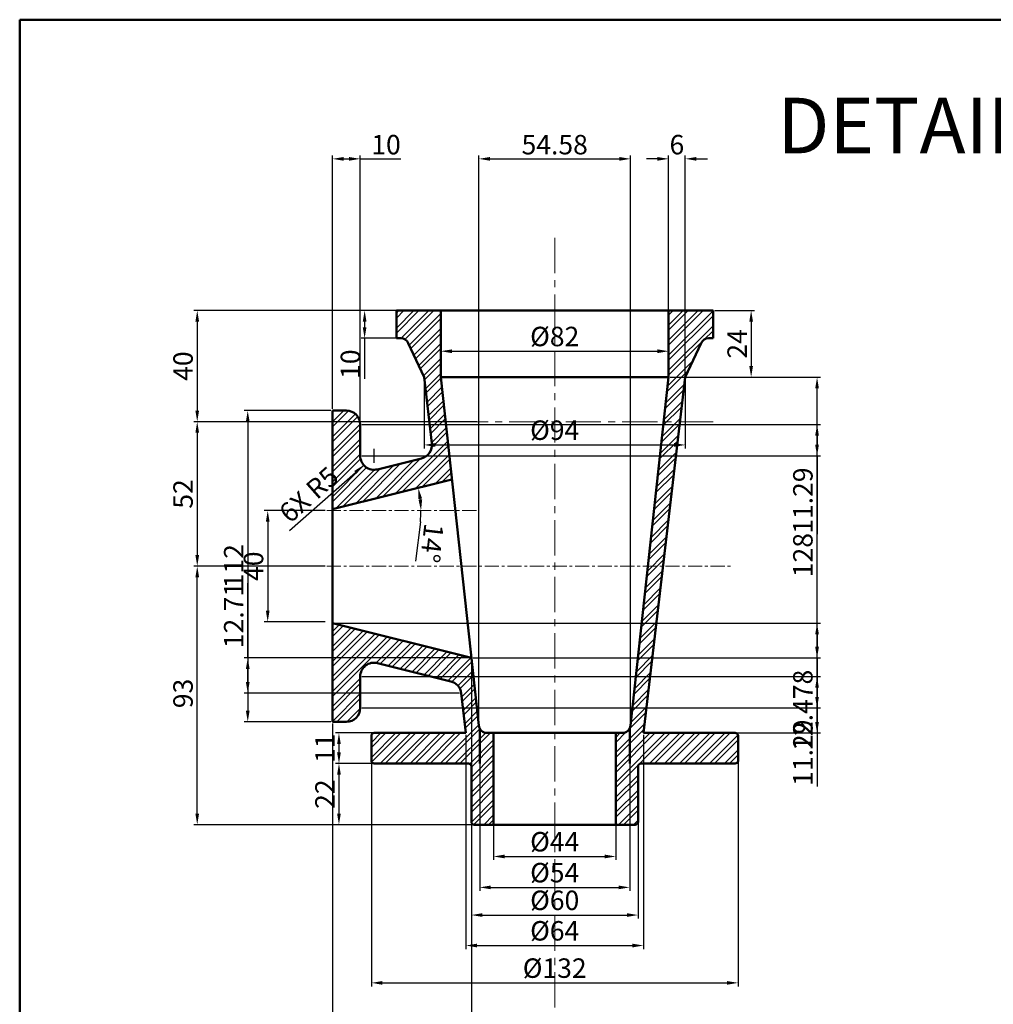
# Model space of a CAD drawing. Units: millimetres. Extents: x 49 to 1001, y -335 to 311.
# Tile 2 of 4: x 49 to 399, y -43 to 311. Entities that reach past the tile are written whole.
import ezdxf

# ---------------------------------------------------------------- set-up
doc = ezdxf.new("R2010")
doc.units = ezdxf.units.MM
doc.header["$LTSCALE"] = 0.4
doc.linetypes.add('CENTER', pattern=[50.8, 31.75, -6.35, 6.35, -6.35])
for name, color, linetype, lineweight in [('M-CNTR', 1, 'CENTER', 18), ('M-DIMS', 2, 'Continuous', 25), ('M-HATC', 8, 'Continuous', 18), ('M-OUTL', 7, 'Continuous', 50), ('M-TEXT', 3, 'Continuous', 25)]:
    doc.layers.add(name, color=color, linetype=linetype, lineweight=lineweight)
doc.styles.get("Standard").update_dxf_attribs({"font": 'arial.ttf'})
doc.dimstyles.new('ISO-25', dxfattribs={"dimtxt": 7, "dimasz": 4, "dimexe": 1.25, "dimexo": 0.625, "dimtad": 1, "dimtxsty": 'Standard', "dimcen": 2.5, "dimadec": 0, "dimazin": 0, "dimtfac": 1, "dimtofl": 0, "dimtmove": 0, "dimatfit": 3, "dimfxl": 1, "dimarcsym": 0})

# ---------------------------------------------------------------- blocks, each defined once
blk = doc.blocks.new('*D1')
at = {"layer": 'Defpoints', "color": 0, "transparency": 16777216}
for p in [(219.24, 38.2), (263.24, 38.2), (263.24, 10.26)]:
    blk.add_point(p, dxfattribs=at)
at = {"layer": 'M-DIMS', "color": 0, "lineweight": -2, "transparency": 16777216}
for p, q in [((219.24, 37.58), (219.24, 9.01)), ((263.24, 37.58), (263.24, 9.01)), ((223.24, 10.26), (259.24, 10.26))]:
    blk.add_line(p, q, dxfattribs=at)
at = {"layer": 'M-DIMS', "color": 0, "transparency": 16777216}
for points in [[(223.24, 10.93), (223.24, 9.59), (219.24, 10.26)], [(259.24, 10.93), (259.24, 9.59), (263.24, 10.26)]]:
    blk.add_solid(points, dxfattribs=at)
at = {"layer": 'M-DIMS', "color": 0, "transparency": 16777216, "insert": (241.24, 14.66), "char_height": 7, "attachment_point": 5}
blk.add_mtext('%%C44', dxfattribs=at)
blk = doc.blocks.new('*D2')
at = {"layer": 'Defpoints', "color": 0, "transparency": 16777216}
for p in [(214.24, 50.04), (268.24, 50.04), (268.24, -0.86)]:
    blk.add_point(p, dxfattribs=at)
at = {"layer": 'M-DIMS', "color": 0, "lineweight": -2, "transparency": 16777216}
for p, q in [((214.24, 49.41), (214.24, -2.11)), ((268.24, 49.41), (268.24, -2.11)), ((218.24, -0.86), (264.24, -0.86))]:
    blk.add_line(p, q, dxfattribs=at)
at = {"layer": 'M-DIMS', "color": 0, "transparency": 16777216}
for points in [[(218.24, -0.19), (218.24, -1.52), (214.24, -0.86)], [(264.24, -0.19), (264.24, -1.52), (268.24, -0.86)]]:
    blk.add_solid(points, dxfattribs=at)
at = {"layer": 'M-DIMS', "color": 0, "transparency": 16777216, "insert": (241.24, 3.54), "char_height": 7, "attachment_point": 5}
blk.add_mtext('%%C54', dxfattribs=at)
blk = doc.blocks.new('*D3')
at = {"layer": 'Defpoints', "color": 0, "transparency": 16777216}
for p in [(209.24, 54.7), (273.24, 54.7), (273.24, -21.78)]:
    blk.add_point(p, dxfattribs=at)
at = {"layer": 'M-DIMS', "color": 0, "lineweight": -2, "transparency": 16777216}
for p, q in [((209.24, 54.08), (209.24, -23.03)), ((273.24, 54.08), (273.24, -23.03)), ((213.24, -21.78), (269.24, -21.78))]:
    blk.add_line(p, q, dxfattribs=at)
at = {"layer": 'M-DIMS', "color": 0, "transparency": 16777216}
for points in [[(213.24, -21.12), (213.24, -22.45), (209.24, -21.78)], [(269.24, -21.12), (269.24, -22.45), (273.24, -21.78)]]:
    blk.add_solid(points, dxfattribs=at)
at = {"layer": 'M-DIMS', "color": 0, "transparency": 16777216, "insert": (241.24, -17.39), "char_height": 7, "attachment_point": 5}
blk.add_mtext('%%C64', dxfattribs=at)
blk = doc.blocks.new('*D4')
at = {"layer": 'Defpoints', "color": 0, "ltscale": 0.4, "transparency": 16777216}
for p in [(211.24, 25.13), (271.24, 25.13), (271.24, -10.81)]:
    blk.add_point(p, dxfattribs=at)
at = {"layer": 'M-DIMS', "color": 0, "lineweight": -2, "ltscale": 0.4, "transparency": 16777216}
for p, q in [((211.24, 24.51), (211.24, -12.06)), ((271.24, 24.51), (271.24, -12.06)), ((215.24, -10.81), (267.24, -10.81))]:
    blk.add_line(p, q, dxfattribs=at)
at = {"layer": 'M-DIMS', "color": 0, "ltscale": 0.4, "transparency": 16777216}
for points in [[(215.24, -10.15), (215.24, -11.48), (211.24, -10.81)], [(267.24, -10.15), (267.24, -11.48), (271.24, -10.81)]]:
    blk.add_solid(points, dxfattribs=at)
at = {"layer": 'M-DIMS', "color": 0, "ltscale": 0.4, "transparency": 16777216, "insert": (241.24, -6.42), "char_height": 7, "attachment_point": 5}
blk.add_mtext('%%C60', dxfattribs=at)
blk = doc.blocks.new('*D5')
at = {"layer": 'Defpoints', "color": 0, "ltscale": 0.4, "transparency": 16777216}
for p in [(175.24, 49.2), (307.24, 49.2), (307.24, -35.21)]:
    blk.add_point(p, dxfattribs=at)
at = {"layer": 'M-DIMS', "color": 0, "lineweight": -2, "ltscale": 0.4, "transparency": 16777216}
for p, q in [((175.24, 48.58), (175.24, -36.46)), ((307.24, 48.58), (307.24, -36.46)), ((179.24, -35.21), (303.24, -35.21))]:
    blk.add_line(p, q, dxfattribs=at)
at = {"layer": 'M-DIMS', "color": 0, "ltscale": 0.4, "transparency": 16777216}
for points in [[(179.24, -34.55), (179.24, -35.88), (175.24, -35.21)], [(303.24, -34.55), (303.24, -35.88), (307.24, -35.21)]]:
    blk.add_solid(points, dxfattribs=at)
at = {"layer": 'M-DIMS', "color": 0, "ltscale": 0.4, "transparency": 16777216, "insert": (241.24, -30.82), "char_height": 7, "attachment_point": 5}
blk.add_mtext('%%C132', dxfattribs=at)
blk = doc.blocks.new('*D6')
at = {"layer": 'Defpoints', "color": 0, "ltscale": 0.4, "transparency": 16777216}
for p in [(180.07, 54.7), (163.58, 43.7), (180.07, 43.7)]:
    blk.add_point(p, dxfattribs=at)
at = {"layer": 'M-DIMS', "color": 0, "lineweight": -2, "ltscale": 0.4, "transparency": 16777216}
for p, q in [((179.45, 54.7), (162.33, 54.7)), ((163.58, 50.7), (163.58, 47.7)), ((179.45, 43.7), (162.33, 43.7))]:
    blk.add_line(p, q, dxfattribs=at)
at = {"layer": 'M-DIMS', "color": 0, "ltscale": 0.4, "transparency": 16777216}
for points in [[(162.91, 50.7), (164.25, 50.7), (163.58, 54.7)], [(162.91, 47.7), (164.25, 47.7), (163.58, 43.7)]]:
    blk.add_solid(points, dxfattribs=at)
at = {"layer": 'M-DIMS', "color": 0, "ltscale": 0.4, "transparency": 16777216, "insert": (159.44, 49.2), "char_height": 7, "attachment_point": 5, "rotation": 90}
blk.add_mtext('11', dxfattribs=at)
blk = doc.blocks.new('*D7')
at = {"layer": 'Defpoints', "color": 0, "ltscale": 0.4, "transparency": 16777216}
for p in [(188.47, 43.7), (163.58, 21.7), (222.94, 21.7)]:
    blk.add_point(p, dxfattribs=at)
at = {"layer": 'M-DIMS', "color": 0, "lineweight": -2, "ltscale": 0.4, "transparency": 16777216}
for p, q in [((187.84, 43.7), (162.33, 43.7)), ((163.58, 39.7), (163.58, 25.7)), ((222.32, 21.7), (162.33, 21.7))]:
    blk.add_line(p, q, dxfattribs=at)
at = {"layer": 'M-DIMS', "color": 0, "ltscale": 0.4, "transparency": 16777216}
for points in [[(162.91, 39.7), (164.25, 39.7), (163.58, 43.7)], [(162.91, 25.7), (164.25, 25.7), (163.58, 21.7)]]:
    blk.add_solid(points, dxfattribs=at)
at = {"layer": 'M-DIMS', "color": 0, "ltscale": 0.4, "transparency": 16777216, "insert": (159.44, 32.7), "char_height": 7, "attachment_point": 5, "rotation": 90}
blk.add_mtext('22', dxfattribs=at)
blk = doc.blocks.new('*D8')
at = {"layer": 'Defpoints', "color": 0, "ltscale": 0.4, "transparency": 16777216}
for p in [(298.24, 206.7), (282.24, 182.7), (311.96, 182.7)]:
    blk.add_point(p, dxfattribs=at)
at = {"layer": 'M-DIMS', "color": 0, "lineweight": -2, "ltscale": 0.4, "transparency": 16777216}
for p, q in [((298.86, 206.7), (313.21, 206.7)), ((311.96, 202.7), (311.96, 186.7)), ((282.86, 182.7), (313.21, 182.7))]:
    blk.add_line(p, q, dxfattribs=at)
at = {"layer": 'M-DIMS', "color": 0, "ltscale": 0.4, "transparency": 16777216}
for points in [[(311.3, 202.7), (312.63, 202.7), (311.96, 206.7)], [(311.3, 186.7), (312.63, 186.7), (311.96, 182.7)]]:
    blk.add_solid(points, dxfattribs=at)
at = {"layer": 'M-DIMS', "color": 0, "ltscale": 0.4, "transparency": 16777216, "insert": (307.82, 194.7), "char_height": 7, "attachment_point": 5, "rotation": 90}
blk.add_mtext('24', dxfattribs=at)
blk = doc.blocks.new('*D9')
at = {"layer": 'Defpoints', "color": 0, "ltscale": 0.4, "transparency": 16777216}
for p in [(200.24, 194.7), (282.24, 194.7), (282.24, 192.06)]:
    blk.add_point(p, dxfattribs=at)
at = {"layer": 'M-DIMS', "color": 0, "lineweight": -2, "ltscale": 0.4, "transparency": 16777216}
for p, q in [((200.24, 194.08), (200.24, 190.81)), ((204.24, 192.06), (278.24, 192.06)), ((282.24, 194.08), (282.24, 190.81))]:
    blk.add_line(p, q, dxfattribs=at)
at = {"layer": 'M-DIMS', "color": 0, "ltscale": 0.4, "transparency": 16777216}
for points in [[(204.24, 192.72), (204.24, 191.39), (200.24, 192.06)], [(278.24, 192.72), (278.24, 191.39), (282.24, 192.06)]]:
    blk.add_solid(points, dxfattribs=at)
at = {"layer": 'M-DIMS', "color": 0, "ltscale": 0.4, "transparency": 16777216, "insert": (241.24, 196.45), "char_height": 7, "attachment_point": 5}
blk.add_mtext('%%C82', dxfattribs=at)
blk = doc.blocks.new('*D10')
at = {"layer": 'Defpoints', "color": 0, "ltscale": 0.4, "transparency": 16777216}
for p in [(184.24, 206.7), (172.82, 196.7), (185.03, 196.7)]:
    blk.add_point(p, dxfattribs=at)
at = {"layer": 'M-DIMS', "color": 0, "lineweight": -2, "ltscale": 0.4, "transparency": 16777216}
for p, q in [((183.61, 206.7), (171.57, 206.7)), ((172.82, 202.7), (172.82, 200.7)), ((184.4, 196.7), (171.57, 196.7)), ((172.82, 196.7), (172.82, 182.11))]:
    blk.add_line(p, q, dxfattribs=at)
at = {"layer": 'M-DIMS', "color": 0, "ltscale": 0.4, "transparency": 16777216}
for points in [[(172.15, 202.7), (173.49, 202.7), (172.82, 206.7)], [(172.15, 200.7), (173.49, 200.7), (172.82, 196.7)]]:
    blk.add_solid(points, dxfattribs=at)
at = {"layer": 'M-DIMS', "color": 0, "ltscale": 0.4, "transparency": 16777216, "insert": (168.62, 187.4), "char_height": 7, "attachment_point": 5, "rotation": 90}
blk.add_mtext('10', dxfattribs=at)
blk = doc.blocks.new('*D11')
at = {"layer": 'Defpoints', "color": 0, "ltscale": 0.4, "transparency": 16777216}
for p in [(213.89, 206.7), (112.56, 166.7), (213.89, 166.7)]:
    blk.add_point(p, dxfattribs=at)
at = {"layer": 'M-DIMS', "color": 0, "lineweight": -2, "ltscale": 0.4, "transparency": 16777216}
for p, q in [((213.27, 206.7), (111.31, 206.7)), ((112.56, 202.7), (112.56, 170.7)), ((213.27, 166.7), (111.31, 166.7))]:
    blk.add_line(p, q, dxfattribs=at)
at = {"layer": 'M-DIMS', "color": 0, "ltscale": 0.4, "transparency": 16777216}
for points in [[(111.9, 202.7), (113.23, 202.7), (112.56, 206.7)], [(111.9, 170.7), (113.23, 170.7), (112.56, 166.7)]]:
    blk.add_solid(points, dxfattribs=at)
at = {"layer": 'M-DIMS', "color": 0, "ltscale": 0.4, "transparency": 16777216, "insert": (108.37, 186.7), "char_height": 7, "attachment_point": 5, "rotation": 90}
blk.add_mtext('40', dxfattribs=at)
blk = doc.blocks.new('*D12')
at = {"layer": 'Defpoints', "color": 0, "ltscale": 0.4, "transparency": 16777216}
for p in [(154.21, 166.7), (112.56, 114.7), (159.19, 114.7)]:
    blk.add_point(p, dxfattribs=at)
at = {"layer": 'M-DIMS', "color": 0, "lineweight": -2, "ltscale": 0.4, "transparency": 16777216}
for p, q in [((153.59, 166.7), (111.31, 166.7)), ((112.56, 162.7), (112.56, 118.7)), ((158.57, 114.7), (111.31, 114.7))]:
    blk.add_line(p, q, dxfattribs=at)
at = {"layer": 'M-DIMS', "color": 0, "ltscale": 0.4, "transparency": 16777216}
for points in [[(111.9, 162.7), (113.23, 162.7), (112.56, 166.7)], [(111.9, 118.7), (113.23, 118.7), (112.56, 114.7)]]:
    blk.add_solid(points, dxfattribs=at)
at = {"layer": 'M-DIMS', "color": 0, "ltscale": 0.4, "transparency": 16777216, "insert": (108.37, 140.7), "char_height": 7, "attachment_point": 5, "rotation": 90}
blk.add_mtext('52', dxfattribs=at)
blk = doc.blocks.new('*D13')
at = {"layer": 'Defpoints', "color": 0, "ltscale": 0.4, "transparency": 16777216}
for p in [(112.56, 114.7), (151.74, 114.7), (175.24, 21.7)]:
    blk.add_point(p, dxfattribs=at)
at = {"layer": 'M-DIMS', "color": 0, "lineweight": -2, "ltscale": 0.4, "transparency": 16777216}
for p, q in [((151.11, 114.7), (111.31, 114.7)), ((112.56, 25.7), (112.56, 110.7)), ((174.61, 21.7), (111.31, 21.7))]:
    blk.add_line(p, q, dxfattribs=at)
at = {"layer": 'M-DIMS', "color": 0, "ltscale": 0.4, "transparency": 16777216}
for points in [[(111.9, 110.7), (113.23, 110.7), (112.56, 114.7)], [(111.9, 25.7), (113.23, 25.7), (112.56, 21.7)]]:
    blk.add_solid(points, dxfattribs=at)
at = {"layer": 'M-DIMS', "color": 0, "ltscale": 0.4, "transparency": 16777216, "insert": (108.36, 68.92), "char_height": 7, "attachment_point": 5, "rotation": 90}
blk.add_mtext('93', dxfattribs=at)
blk = doc.blocks.new('*D14')
at = {"layer": 'Defpoints', "color": 0, "ltscale": 0.4, "transparency": 16777216}
for p in [(194.24, 182.7), (288.24, 182.7), (288.24, 158.34)]:
    blk.add_point(p, dxfattribs=at)
at = {"layer": 'M-DIMS', "color": 0, "lineweight": -2, "ltscale": 0.4, "transparency": 16777216}
for p, q in [((194.24, 182.08), (194.24, 157.09)), ((288.24, 182.08), (288.24, 157.09)), ((198.24, 158.34), (284.24, 158.34))]:
    blk.add_line(p, q, dxfattribs=at)
at = {"layer": 'M-DIMS', "color": 0, "ltscale": 0.4, "transparency": 16777216}
for points in [[(198.24, 159.01), (198.24, 157.67), (194.24, 158.34)], [(284.24, 159.01), (284.24, 157.67), (288.24, 158.34)]]:
    blk.add_solid(points, dxfattribs=at)
at = {"layer": 'M-DIMS', "color": 0, "ltscale": 0.4, "transparency": 16777216, "insert": (241.24, 162.74), "char_height": 7, "attachment_point": 5}
blk.add_mtext('%%C94', dxfattribs=at)
blk = doc.blocks.new('*D15')
at = {"layer": 'Defpoints', "color": 0, "ltscale": 0.4, "transparency": 16777216}
for p in [(159.19, 134.7), (137.93, 94.7), (159.19, 94.7)]:
    blk.add_point(p, dxfattribs=at)
at = {"layer": 'M-DIMS', "color": 0, "lineweight": -2, "ltscale": 0.4, "transparency": 16777216}
for p, q in [((158.57, 134.7), (136.68, 134.7)), ((137.93, 130.7), (137.93, 98.7)), ((158.57, 94.7), (136.68, 94.7))]:
    blk.add_line(p, q, dxfattribs=at)
at = {"layer": 'M-DIMS', "color": 0, "ltscale": 0.4, "transparency": 16777216}
for points in [[(137.27, 130.7), (138.6, 130.7), (137.93, 134.7)], [(137.27, 98.7), (138.6, 98.7), (137.93, 94.7)]]:
    blk.add_solid(points, dxfattribs=at)
at = {"layer": 'M-DIMS', "color": 0, "ltscale": 0.4, "transparency": 16777216, "insert": (133.73, 114.7), "char_height": 7, "attachment_point": 5, "rotation": 90}
blk.add_mtext('40', dxfattribs=at)
blk = doc.blocks.new('*D16')
at = {"layer": 'Defpoints', "color": 0, "ltscale": 0.4, "transparency": 16777216}
for p in [(204.26, 145.94), (192.66, 140.2), (159.19, 134.7), (159.19, 134.7), (213.55, 134.7)]:
    blk.add_point(p, dxfattribs=at)
at = {"layer": 'M-DIMS', "color": 0, "lineweight": -2, "ltscale": 0.4, "transparency": 16777216}
blk.add_line((192.88, 130.71), (191.19, 116.48), dxfattribs=at)
for start, end in [(6.7604, 7.2396), (353.2396, 360)]:
    blk.add_arc((159.19, 134.7), 33.92, start, end, dxfattribs=at)
at = {"layer": 'M-DIMS', "color": 0, "ltscale": 0.4, "transparency": 16777216}
for points in [[(192.19, 138.85), (193.5, 139.1), (192.11, 142.91)], [(193.54, 138.73), (192.21, 138.66), (193.11, 134.7)]]:
    blk.add_solid(points, dxfattribs=at)
at = {"layer": 'M-DIMS', "color": 0, "ltscale": 0.4, "transparency": 16777216, "insert": (196.14, 123.11), "char_height": 7, "attachment_point": 5, "rotation": 263.2396}
blk.add_mtext('14°', dxfattribs=at)
blk = doc.blocks.new('*D58')
at = {"layer": 'Defpoints', "color": 0, "ltscale": 0.4, "transparency": 16777216}
for p in [(211.28, 81.71), (161.24, 58.7), (211.28, -274.62)]:
    blk.add_point(p, dxfattribs=at)
at = {"layer": 'M-DIMS', "color": 0, "lineweight": -2, "ltscale": 0.4, "transparency": 16777216}
for p, q in [((211.28, 81.09), (211.28, -275.87)), ((161.24, 58.08), (161.24, -275.87)), ((165.24, -274.62), (207.28, -274.62))]:
    blk.add_line(p, q, dxfattribs=at)
at = {"layer": 'M-DIMS', "color": 0, "ltscale": 0.4, "transparency": 16777216}
for points in [[(165.24, -273.95), (165.24, -275.28), (161.24, -274.62)], [(207.28, -273.95), (207.28, -275.28), (211.28, -274.62)]]:
    blk.add_solid(points, dxfattribs=at)
at = {"layer": 'M-DIMS', "color": 0, "ltscale": 0.4, "transparency": 16777216, "insert": (186.26, -270.42), "char_height": 7, "attachment_point": 5}
blk.add_mtext('50.05', dxfattribs=at)
blk = doc.blocks.new('*D59')
at = {"layer": 'Defpoints', "color": 0, "ltscale": 0.4, "transparency": 16777216}
for p in [(161.24, 94.19), (211.28, 81.71), (335.69, 81.71)]:
    blk.add_point(p, dxfattribs=at)
at = {"layer": 'M-DIMS', "color": 0, "lineweight": -2, "ltscale": 0.4, "transparency": 16777216}
for p, q in [((161.86, 94.19), (336.94, 94.19)), ((335.69, 90.19), (335.69, 85.71)), ((211.91, 81.71), (336.94, 81.71)), ((335.69, 81.71), (335.69, 48.05))]:
    blk.add_line(p, q, dxfattribs=at)
at = {"layer": 'M-DIMS', "color": 0, "ltscale": 0.4, "transparency": 16777216}
for points in [[(335.02, 90.19), (336.35, 90.19), (335.69, 94.19)], [(335.02, 85.71), (336.35, 85.71), (335.69, 81.71)]]:
    blk.add_solid(points, dxfattribs=at)
at = {"layer": 'M-DIMS', "color": 0, "ltscale": 0.4, "transparency": 16777216, "insert": (331.49, 62.88), "char_height": 7, "attachment_point": 5, "rotation": 90}
blk.add_mtext('12.478', dxfattribs=at)
blk = doc.blocks.new('*D60')
at = {"layer": 'Defpoints', "color": 0, "ltscale": 0.4, "transparency": 16777216}
for p in [(130.74, 81.71), (211.28, 81.71), (207.56, 69)]:
    blk.add_point(p, dxfattribs=at)
at = {"layer": 'M-DIMS', "color": 0, "lineweight": -2, "ltscale": 0.4, "transparency": 16777216}
for p, q in [((130.74, 81.71), (130.74, 108.58)), ((210.66, 81.71), (129.49, 81.71)), ((130.74, 73), (130.74, 77.71)), ((206.94, 69), (129.49, 69))]:
    blk.add_line(p, q, dxfattribs=at)
at = {"layer": 'M-DIMS', "color": 0, "ltscale": 0.4, "transparency": 16777216}
for points in [[(130.08, 77.71), (131.41, 77.71), (130.74, 81.71)], [(130.08, 73), (131.41, 73), (130.74, 69)]]:
    blk.add_solid(points, dxfattribs=at)
at = {"layer": 'M-DIMS', "color": 0, "ltscale": 0.4, "transparency": 16777216, "insert": (126.6, 97.14), "char_height": 7, "attachment_point": 5, "rotation": 90}
blk.add_mtext('12.71', dxfattribs=at)
blk = doc.blocks.new('*D61')
at = {"layer": 'Defpoints', "color": 0, "ltscale": 0.4, "transparency": 16777216}
for p in [(161.24, 170.7), (130.74, 58.7), (161.24, 58.7)]:
    blk.add_point(p, dxfattribs=at)
at = {"layer": 'M-DIMS', "color": 0, "lineweight": -2, "ltscale": 0.4, "transparency": 16777216}
for p, q in [((160.61, 170.7), (129.49, 170.7)), ((130.74, 166.7), (130.74, 62.7)), ((160.61, 58.7), (129.49, 58.7))]:
    blk.add_line(p, q, dxfattribs=at)
at = {"layer": 'M-DIMS', "color": 0, "ltscale": 0.4, "transparency": 16777216}
for points in [[(130.08, 166.7), (131.41, 166.7), (130.74, 170.7)], [(130.08, 62.7), (131.41, 62.7), (130.74, 58.7)]]:
    blk.add_solid(points, dxfattribs=at)
at = {"layer": 'M-DIMS', "color": 0, "ltscale": 0.4, "transparency": 16777216, "insert": (126.6, 114.7), "char_height": 7, "attachment_point": 5, "rotation": 90}
blk.add_mtext('112', dxfattribs=at)
blk = doc.blocks.new('*D62')
at = {"layer": 'Defpoints', "color": 0, "ltscale": 0.4, "transparency": 16777216}
for p in [(171.24, 261.28), (161.24, 170.7), (171.24, 165.7)]:
    blk.add_point(p, dxfattribs=at)
at = {"layer": 'M-DIMS', "color": 0, "lineweight": -2, "ltscale": 0.4, "transparency": 16777216}
for p, q in [((161.24, 171.33), (161.24, 262.53)), ((171.24, 166.33), (171.24, 262.53)), ((165.24, 261.28), (167.24, 261.28)), ((171.24, 261.28), (185.83, 261.28))]:
    blk.add_line(p, q, dxfattribs=at)
at = {"layer": 'M-DIMS', "color": 0, "ltscale": 0.4, "transparency": 16777216}
for points in [[(165.24, 261.94), (165.24, 260.61), (161.24, 261.28)], [(167.24, 261.94), (167.24, 260.61), (171.24, 261.28)]]:
    blk.add_solid(points, dxfattribs=at)
at = {"layer": 'M-DIMS', "color": 0, "ltscale": 0.4, "transparency": 16777216, "insert": (180.53, 265.48), "char_height": 7, "attachment_point": 5}
blk.add_mtext('10', dxfattribs=at)
blk = doc.blocks.new('*D63')
at = {"layer": 'Defpoints', "color": 0, "ltscale": 0.4, "transparency": 16777216}
for p in [(171.24, 165.7), (171.24, 154.41), (335.69, 154.41)]:
    blk.add_point(p, dxfattribs=at)
at = {"layer": 'M-DIMS', "color": 0, "lineweight": -2, "ltscale": 0.4, "transparency": 16777216}
for p, q in [((171.86, 165.7), (336.94, 165.7)), ((335.69, 161.7), (335.69, 158.41)), ((171.86, 154.41), (336.94, 154.41)), ((335.69, 154.41), (335.69, 126.18))]:
    blk.add_line(p, q, dxfattribs=at)
at = {"layer": 'M-DIMS', "color": 0, "ltscale": 0.4, "transparency": 16777216}
for points in [[(335.02, 161.7), (336.35, 161.7), (335.69, 165.7)], [(335.02, 158.41), (336.35, 158.41), (335.69, 154.41)]]:
    blk.add_solid(points, dxfattribs=at)
at = {"layer": 'M-DIMS', "color": 0, "ltscale": 0.4, "transparency": 16777216, "insert": (331.49, 138.3), "char_height": 7, "attachment_point": 5, "rotation": 90}
blk.add_mtext('11.29', dxfattribs=at)
blk = doc.blocks.new('*D64')
at = {"layer": 'Defpoints', "color": 0, "ltscale": 0.4, "transparency": 16777216}
for p in [(171.24, 74.99), (171.24, 63.7), (335.69, 63.7)]:
    blk.add_point(p, dxfattribs=at)
at = {"layer": 'M-DIMS', "color": 0, "lineweight": -2, "ltscale": 0.4, "transparency": 16777216}
for p, q in [((171.86, 74.99), (336.94, 74.99)), ((335.69, 70.99), (335.69, 67.7)), ((171.86, 63.7), (336.94, 63.7)), ((335.69, 63.7), (335.69, 35.48))]:
    blk.add_line(p, q, dxfattribs=at)
at = {"layer": 'M-DIMS', "color": 0, "ltscale": 0.4, "transparency": 16777216}
for points in [[(335.02, 70.99), (336.35, 70.99), (335.69, 74.99)], [(335.02, 67.7), (336.35, 67.7), (335.69, 63.7)]]:
    blk.add_solid(points, dxfattribs=at)
at = {"layer": 'M-DIMS', "color": 0, "ltscale": 0.4, "transparency": 16777216, "insert": (331.49, 47.59), "char_height": 7, "attachment_point": 5, "rotation": 90}
blk.add_mtext('11.29', dxfattribs=at)
blk = doc.blocks.new('*D65')
at = {"layer": 'Defpoints', "color": 0, "ltscale": 0.4, "transparency": 16777216}
for p in [(288.24, 261.28), (282.24, 182.7), (288.24, 182.7)]:
    blk.add_point(p, dxfattribs=at)
at = {"layer": 'M-DIMS', "color": 0, "lineweight": -2, "ltscale": 0.4, "transparency": 16777216}
for p, q in [((282.24, 183.33), (282.24, 262.53)), ((288.24, 183.33), (288.24, 262.53)), ((278.24, 261.28), (274.24, 261.28)), ((292.24, 261.28), (296.24, 261.28))]:
    blk.add_line(p, q, dxfattribs=at)
at = {"layer": 'M-DIMS', "color": 0, "ltscale": 0.4, "transparency": 16777216}
for points in [[(278.24, 261.94), (278.24, 260.61), (282.24, 261.28)], [(292.24, 261.94), (292.24, 260.61), (288.24, 261.28)]]:
    blk.add_solid(points, dxfattribs=at)
at = {"layer": 'M-DIMS', "color": 0, "ltscale": 0.4, "transparency": 16777216, "insert": (285.24, 265.48), "char_height": 7, "attachment_point": 5}
blk.add_mtext('6', dxfattribs=at)
blk = doc.blocks.new('*D66')
at = {"layer": 'Defpoints', "color": 0, "ltscale": 0.4, "transparency": 16777216}
for p in [(268.53, 261.28), (213.94, 57.38), (268.53, 57.38)]:
    blk.add_point(p, dxfattribs=at)
at = {"layer": 'M-DIMS', "color": 0, "lineweight": -2, "ltscale": 0.4, "transparency": 16777216}
for p, q in [((213.94, 58), (213.94, 262.53)), ((268.53, 58), (268.53, 262.53)), ((217.94, 261.28), (264.53, 261.28))]:
    blk.add_line(p, q, dxfattribs=at)
at = {"layer": 'M-DIMS', "color": 0, "ltscale": 0.4, "transparency": 16777216}
for points in [[(217.94, 261.94), (217.94, 260.61), (213.94, 261.28)], [(264.53, 261.94), (264.53, 260.61), (268.53, 261.28)]]:
    blk.add_solid(points, dxfattribs=at)
at = {"layer": 'M-DIMS', "color": 0, "ltscale": 0.4, "transparency": 16777216, "insert": (241.24, 265.48), "char_height": 7, "attachment_point": 5}
blk.add_mtext('54.58', dxfattribs=at)
blk = doc.blocks.new('*D67')
at = {"layer": 'Defpoints', "color": 0, "ltscale": 0.4, "transparency": 16777216}
for p in [(288.24, 182.7), (335.69, 182.7), (273.24, 54.7)]:
    blk.add_point(p, dxfattribs=at)
at = {"layer": 'M-DIMS', "color": 0, "lineweight": -2, "ltscale": 0.4, "transparency": 16777216}
for p, q in [((288.86, 182.7), (336.94, 182.7)), ((335.69, 58.7), (335.69, 178.7)), ((273.86, 54.7), (336.94, 54.7))]:
    blk.add_line(p, q, dxfattribs=at)
at = {"layer": 'M-DIMS', "color": 0, "ltscale": 0.4, "transparency": 16777216}
for points in [[(335.02, 178.7), (336.35, 178.7), (335.69, 182.7)], [(335.02, 58.7), (336.35, 58.7), (335.69, 54.7)]]:
    blk.add_solid(points, dxfattribs=at)
at = {"layer": 'M-DIMS', "color": 0, "ltscale": 0.4, "transparency": 16777216, "insert": (331.49, 118.7), "char_height": 7, "attachment_point": 5, "rotation": 90}
blk.add_mtext('128', dxfattribs=at)
blk = doc.blocks.new('*D71')
at = {"layer": 'Defpoints', "color": 0, "ltscale": 0.4, "transparency": 16777216}
for p in [(176.24, 154.41), (172.49, 151.1)]:
    blk.add_point(p, dxfattribs=at)
at = {"layer": 'M-DIMS', "color": 0, "lineweight": -2, "ltscale": 0.4, "transparency": 16777216}
for p, q in [((176.24, 151.91), (176.24, 156.91)), ((173.74, 154.41), (178.74, 154.41)), ((145.75, 127.5), (169.49, 148.45))]:
    blk.add_line(p, q, dxfattribs=at)
at = {"layer": 'M-DIMS', "color": 0, "ltscale": 0.4, "transparency": 16777216}
blk.add_solid([(169.05, 148.95), (169.93, 147.95), (172.49, 151.1)], dxfattribs=at)
at = {"layer": 'M-DIMS', "color": 0, "ltscale": 0.4, "transparency": 16777216, "insert": (153.34, 139.8), "char_height": 7, "attachment_point": 5, "rotation": 41.4391}
blk.add_mtext('6X R5', dxfattribs=at)

msp = doc.modelspace()

# ---------------------------------------------------------------- hatches: boundary and pattern name
at = {"layer": 'M-HATC', "ltscale": 0.4}
h = msp.add_hatch(dxfattribs=at)
h.set_pattern_fill('ANSI32', color=256, scale=0.4)
h.paths.add_polyline_path([(161.2373, 94.1921), (161.2373, 58.7021), (166.2373, 58.7021, 0.41421356), (171.2373, 63.7021), (171.2373, 74.993, -0.48773259), (177.4469, 79.8444), (203.805, 73.2726, -0.3120213), (207.5614, 69.0031), (209.2373, 54.7021), (176.2373, 54.7021, 0.41421356), (175.2373, 53.7021), (175.2373, 44.7021, 0.41421356), (176.2373, 43.7021), (210.2373, 43.7021, -0.41421356), (211.2373, 42.7021), (211.2373, 22.7021, 0.41421356), (212.2373, 21.7021), (219.2373, 21.7021), (219.2373, 54.7021), (216.9271, 54.7021, -0.38265344), (213.9449, 57.3759), (211.2829, 81.7143)])
h.paths.add_polyline_path([(307.2373, 53.7021, 0.41421356), (306.2373, 54.7021), (273.2373, 54.7021), (280.2686, 114.7021), (274.7998, 114.7021), (268.5298, 57.3759, -0.38265344), (265.5476, 54.7021), (263.2373, 54.7021), (263.2373, 21.7021), (270.2373, 21.7021, 0.41421356), (271.2373, 22.7021), (271.2373, 42.7021, -0.41421356), (272.2373, 43.7021), (306.2373, 43.7021, 0.41421356), (307.2373, 44.7021)])
h.paths.add_polyline_path([(286.3623, 166.7021), (280.4873, 166.7021), (274.7998, 114.7021), (280.2686, 114.7021)])
h.paths.add_polyline_path([(204.2584, 145.9384), (201.9873, 166.7021), (196.1123, 166.7021), (197.0223, 158.9372, -0.37728953), (193.2659, 153.5038), (177.4469, 149.5597, -0.48773259), (171.2373, 154.4111), (171.2373, 165.7021, 0.41421356), (166.2373, 170.7021), (161.2373, 170.7021), (161.2373, 135.212)])
h.paths.add_polyline_path([(200.2373, 206.7021), (184.2373, 206.7021), (184.2373, 196.7021), (185.8226, 196.7021, -0.2919243), (188.5436, 194.9654), (194.2373, 182.7021), (196.1123, 166.7021), (201.9873, 166.7021), (200.2373, 182.7021)])
h.paths.add_polyline_path([(298.2373, 206.7021), (282.2373, 206.7021), (282.2373, 182.7021), (280.4873, 166.7021), (286.3623, 166.7021), (288.2373, 182.7021), (293.931, 194.9654, -0.2919243), (296.652, 196.7021), (298.2373, 196.7021)])

# ---------------------------------------------------------------- linework, layer by layer
at = {"layer": 'M-CNTR'}
for p, q in [((241.2373, 232.8267), (241.2373, -233.1822)), ((184.2373, 166.7021), (298.2373, 166.7021))]:
    msp.add_line(p, q, dxfattribs=at)
at = {"layer": 'M-CNTR', "ltscale": 0.4}
for p, q in [((159.192, 134.7021), (213.5534, 134.7021)), ((159.192, 114.7021), (305.3031, 114.7021))]:
    msp.add_line(p, q, dxfattribs=at)
at = {"layer": 'M-OUTL'}
for p, q in [((184.2373, 206.7021), (298.2373, 206.7021)), ((184.2373, 206.7021), (184.2373, 196.7021)), ((184.2373, 206.7021), (184.2373, 196.7021)), ((200.2373, 206.7021), (200.2373, 182.7021)), ((282.2373, 206.7021), (282.2373, 182.7021)), ((298.2373, 206.7021), (298.2373, 196.7021)), ((184.2373, 196.7021), (185.8226, 196.7021)), ((194.2373, 182.7021), (188.5436, 194.9654)), ((288.2373, 182.7021), (293.931, 194.9654)), ((296.652, 196.7021), (298.2373, 196.7021)), ((197.0223, 158.9372), (194.2373, 182.7021)), ((200.2373, 182.7021), (282.2373, 182.7021)), ((213.9449, 57.3759), (200.2373, 182.7021)), ((282.2373, 182.7021), (268.5298, 57.3759)), ((273.2373, 54.7021), (288.2373, 182.7021)), ((161.2373, 170.7021), (166.2373, 170.7021)), ((161.2373, 170.7021), (161.2373, 58.7021)), ((171.2373, 165.7021), (171.2373, 154.4111)), ((177.4469, 149.5597), (193.2659, 153.5038)), ((161.2373, 135.212), (204.2584, 145.9384)), ((161.2373, 94.1921), (211.2829, 81.7143)), ((177.4469, 79.8444), (203.805, 73.2726)), ((171.2373, 74.993), (171.2373, 63.7021)), ((209.2373, 54.7021), (207.5614, 69.0031)), ((161.2373, 58.7021), (166.2373, 58.7021)), ((175.2373, 44.7021), (175.2373, 53.7021)), ((176.2373, 54.7021), (209.2373, 54.7021)), ((214.2373, 56.3735), (214.2373, 43.7021)), ((216.9271, 54.7021), (265.5476, 54.7021)), ((219.2373, 54.7021), (219.2373, 21.7021)), ((263.2373, 54.7021), (263.2373, 21.7021)), ((268.2373, 56.3735), (268.2373, 43.7021)), ((273.2373, 54.7021), (306.2373, 54.7021)), ((307.2373, 53.7021), (307.2373, 44.7021)), ((210.2373, 43.7021), (176.2373, 43.7021)), ((211.2373, 42.7021), (211.2373, 22.7021)), ((271.2373, 42.7021), (271.2373, 22.7021)), ((306.2373, 43.7021), (272.2373, 43.7021)), ((270.2373, 21.7021), (212.2373, 21.7021))]:
    msp.add_line(p, q, dxfattribs=at)
at = {"layer": 'M-OUTL', "ltscale": 0.4}
msp.add_lwpolyline([(48.6466, 311.3462), (1001.3348, 311.3462), (1001.3348, -335.0483), (48.6466, -335.0483)], close=True, dxfattribs=at)
at = {"layer": 'M-OUTL'}
for centre, radius, start, end in [((185.8226, 193.7021), 3, 24.904769, 90), ((296.652, 193.7021), 3, 90, 155.095231), ((166.2373, 165.7021), 5, 0, 90), ((192.0563, 158.3552), 5, 284, 6.683864), ((176.2373, 154.4111), 5, 180, 284), ((176.2373, 74.993), 5, 76, 180), ((202.5954, 68.4212), 5, 6.683864, 76), ((166.2373, 63.7021), 5, 270, 0), ((216.9271, 57.7021), 3, 186.241914, 270), ((265.5476, 57.7021), 3, 270, 353.758086), ((176.2373, 53.7021), 1, 90, 180), ((306.2373, 53.7021), 1, 0, 90), ((176.2373, 44.7021), 1, 180, 270), ((210.2373, 42.7021), 1, 0, 90), ((272.2373, 42.7021), 1, 90, 180), ((306.2373, 44.7021), 1, 270, 0), ((212.2373, 22.7021), 1, 180, 270), ((270.2373, 22.7021), 1, 270, 0)]:
    msp.add_arc(centre, radius, start, end, dxfattribs=at)

# ---------------------------------------------------------------- texts
at = {"layer": 'M-TEXT', "ltscale": 0.4, "insert": (295.8479, 283.2448), "char_height": 20, "attachment_point": 1}
msp.add_mtext_dynamic_manual_height_columns('\\pxqc;DETAILS OF BLOW OFF COCK', width=417.660537, gutter_width=12.5, heights=[0], dxfattribs=at)

# ---------------------------------------------------------------- dimensions: what is measured, and where the dimension line sits
at = {"layer": 'M-DIMS', "ltscale": 0.4}
for base, p1, p2, override, picture, middle in [((171.2373, 261.2767), (161.2373, 170.7021), (171.2373, 165.7021), {"dimdec": 0, "dimlfac": 1, "dimrnd": 0, "dimzin": 0, "dimdsep": 46, "dimlunit": 2}, '*D62', (180.5346, 265.4757)), ((268.5298, 261.2767), (213.9449, 57.3759), (268.5298, 57.3759), {"dimdec": 2, "dimlfac": 1, "dimrnd": 0, "dimzin": 0, "dimdsep": 46, "dimlunit": 2}, '*D66', (241.2373, 265.4757)), ((288.2373, 261.2767), (282.2373, 182.7021), (288.2373, 182.7021), {"dimdec": 0, "dimlfac": 1, "dimrnd": 0, "dimzin": 0, "dimdsep": 46, "dimlunit": 2}, '*D65', (285.2373, 265.4757)), ((211.2829, -274.6166), (161.2373, 58.7021), (211.2829, 81.7143), {"dimdec": 2, "dimlfac": 1, "dimrnd": 0, "dimzin": 0, "dimdsep": 46, "dimlunit": 2}, '*D58', (186.2601, -270.4176))]:
    dim = msp.add_linear_dim(base=base, p1=p1, p2=p2, dimstyle='ISO-25', override=override, dxfattribs=at)
    dim.commit()
    dim.dimension.update_dxf_attribs({"geometry": picture, "text_midpoint": middle})
for base, p1, p2, override, picture, middle in [((112.5649, 166.7021), (213.8942, 206.7021), (213.8942, 166.7021), {"dimclrd": 0, "dimclre": 0, "dimclrt": 0}, '*D11', (108.3659, 186.7021)), ((172.8207, 196.7021), (184.2373, 206.7021), (185.03, 196.7021), {"dimclrd": 0, "dimclre": 0, "dimclrt": 0}, '*D10', (168.6217, 187.4048)), ((311.9634, 182.7021), (298.2373, 206.7021), (282.2373, 182.7021), {"dimclrd": 0, "dimclre": 0, "dimclrt": 0}, '*D8', (307.824, 194.7021)), ((335.6873, 182.7021), (273.2373, 54.7021), (288.2373, 182.7021), {"dimdec": 0, "dimlfac": 1, "dimrnd": 0, "dimzin": 0, "dimdsep": 46, "dimlunit": 2}, '*D67', (331.4883, 118.7021)), ((130.742, 58.7021), (161.2373, 170.7021), (161.2373, 58.7021), {"dimdec": 0, "dimlfac": 1, "dimrnd": 0, "dimzin": 0, "dimdsep": 46, "dimlunit": 2}, '*D61', (126.6026, 114.7021)), ((112.5649, 114.7021), (154.2122, 166.7021), (159.192, 114.7021), {"dimclrd": 0, "dimclre": 0, "dimclrt": 0}, '*D12', (108.3659, 140.7021)), ((335.6873, 154.4111), (171.2373, 165.7021), (171.2373, 154.4111), {"dimdec": 2, "dimlfac": 1, "dimrnd": 0, "dimzin": 0, "dimdsep": 46, "dimlunit": 2}, '*D63', (331.4883, 138.2977)), ((137.9319, 94.7021), (159.192, 134.7021), (159.192, 94.7021), {"dimclrd": 0, "dimclre": 0, "dimclrt": 0}, '*D15', (133.7329, 114.7021)), ((130.742, 81.7143), (207.5614, 69.0031), (211.2829, 81.7143), {"dimdec": 2, "dimlfac": 1, "dimrnd": 0, "dimzin": 0, "dimdsep": 46, "dimlunit": 2}, '*D60', (126.6026, 97.1449)), ((335.6873, 81.7143), (161.2373, 94.1921), (211.2829, 81.7143), {"dimdec": 3, "dimlfac": 1, "dimrnd": 0, "dimzin": 0, "dimdsep": 46, "dimlunit": 2}, '*D59', (331.4883, 62.8816)), ((335.6873, 63.7021), (171.2373, 74.993), (171.2373, 63.7021), {"dimdec": 2, "dimlfac": 1, "dimrnd": 0, "dimzin": 0, "dimdsep": 46, "dimlunit": 2}, '*D64', (331.4883, 47.5887)), ((163.5804, 43.7021), (180.0736, 54.7021), (180.0736, 43.7021), {"dimclrd": 0, "dimclre": 0, "dimclrt": 0}, '*D6', (159.4411, 49.2021)), ((163.5804, 21.7021), (188.4674, 43.7021), (222.9437, 21.7021), {"dimclrd": 0, "dimclre": 0, "dimclrt": 0}, '*D7', (159.4411, 32.7021))]:
    dim = msp.add_linear_dim(base=base, p1=p1, p2=p2, angle=90, dimstyle='ISO-25', override=override, dxfattribs=at)
    dim.commit()
    dim.dimension.update_dxf_attribs({"geometry": picture, "text_midpoint": middle})
for base, p1, p2, picture, middle in [((282.2373, 192.0551), (200.2373, 194.7021), (282.2373, 194.7021), '*D9', (241.2373, 196.4499)), ((288.2373, 158.341), (194.2373, 182.7021), (288.2373, 182.7021), '*D14', (241.2373, 162.7358)), ((307.2373, -35.2133), (175.2373, 49.2021), (307.2373, 49.2021), '*D5', (241.2373, -30.8185))]:
    dim = msp.add_linear_dim(base=base, p1=p1, p2=p2, text='%%C<>', dimstyle='ISO-25', override={"dimclrd": 0, "dimclre": 0, "dimclrt": 0}, dxfattribs=at)
    dim.commit()
    dim.dimension.update_dxf_attribs({"geometry": picture, "text_midpoint": middle})
dim = msp.add_radius_dim(center=(176.2373, 154.4111), mpoint=(172.489, 151.102), text='6X <>', dimstyle='ISO-25', override={"dimdec": 0, "dimlfac": 1, "dimrnd": 0, "dimzin": 0, "dimdsep": 46, "dimlunit": 2}, dxfattribs=at)
dim.commit()
dim.dimension.update_dxf_attribs({"geometry": '*D71', "text_midpoint": (153.3414, 139.7991)})
dim = msp.add_angular_dim_2l(base=(192.6636, 140.2032), line1=((159.192, 134.7021), (213.5534, 134.7021)), line2=((159.192, 134.7021), (204.2584, 145.9384)), dimstyle='ISO-25', override={"dimclrd": 0, "dimclre": 0, "dimclrt": 0}, dxfattribs=at)
dim.commit()
dim.dimension.update_dxf_attribs({"geometry": '*D16', "text_midpoint": (196.1443, 123.1097)})
dim = msp.add_linear_dim(base=(112.5649, 114.7021), p1=(175.2373, 21.7021), p2=(151.7367, 114.7021), angle=90, dimstyle='ISO-25', override={"dimclrd": 0, "dimclre": 0, "dimclrt": 0}, dxfattribs=at)
dim.commit()
dim.dimension.update_dxf_attribs({"geometry": '*D13', "text_midpoint": (112.5649, 68.9237), "dimtype": 160})
at = {"layer": 'M-DIMS'}
dim = msp.add_linear_dim(base=(273.2373, -21.7841), p1=(209.2373, 54.7021), p2=(273.2373, 54.7021), text='%%C<>', dimstyle='ISO-25', override={"dimclrd": 0, "dimclre": 0, "dimclrt": 0}, dxfattribs=at)
dim.commit()
dim.dimension.update_dxf_attribs({"geometry": '*D3', "text_midpoint": (241.2373, -21.7841), "dimtype": 160})
for base, p1, p2, picture, middle in [((268.2373, -0.8558), (214.2373, 50.0378), (268.2373, 50.0378), '*D2', (241.2373, 3.539)), ((263.2373, 10.2604), (219.2373, 38.2021), (263.2373, 38.2021), '*D1', (241.2373, 14.6552))]:
    dim = msp.add_linear_dim(base=base, p1=p1, p2=p2, text='%%C<>', dimstyle='ISO-25', override={"dimclrd": 0, "dimclre": 0, "dimclrt": 0}, dxfattribs=at)
    dim.commit()
    dim.dimension.update_dxf_attribs({"geometry": picture, "text_midpoint": middle})
at = {"layer": 'M-DIMS', "ltscale": 0.4}
dim = msp.add_linear_dim(base=(271.2373, -10.8137), p1=(211.2373, 25.1322), p2=(271.2373, 25.1322), text='%%C<>', dimstyle='ISO-25', override={"dimclrd": 0, "dimclre": 0, "dimclrt": 0}, dxfattribs=at)
dim.commit()
dim.dimension.update_dxf_attribs({"geometry": '*D4', "text_midpoint": (241.2373, -10.8137), "dimtype": 160})

doc.saveas('drawing.dxf')
